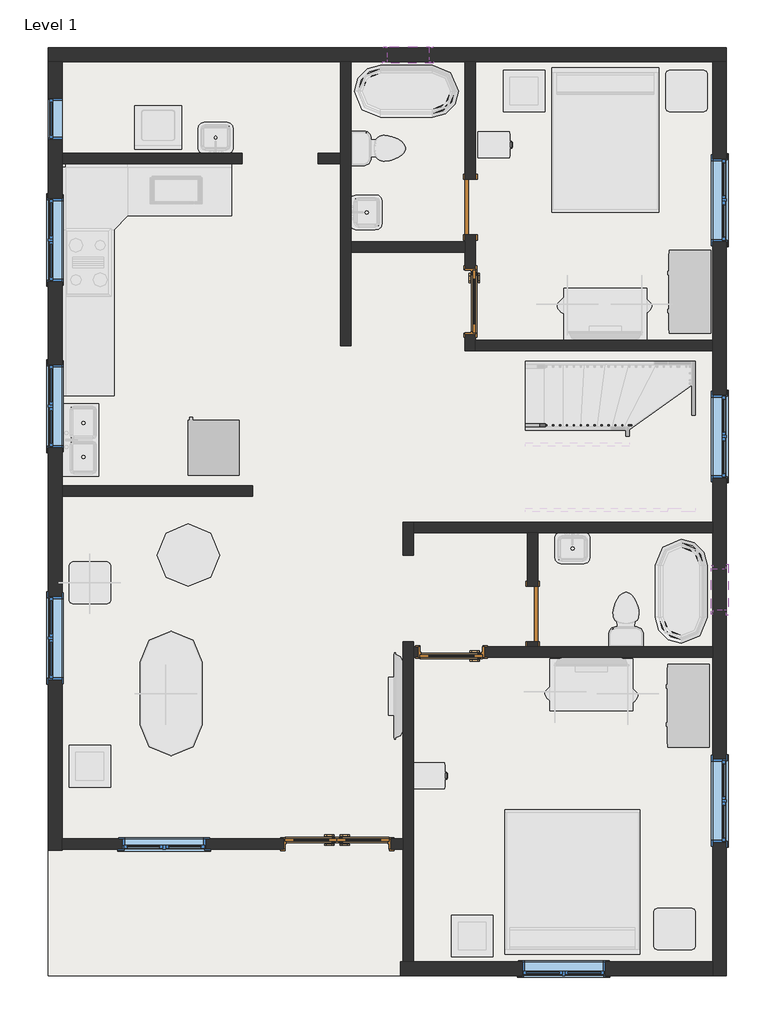
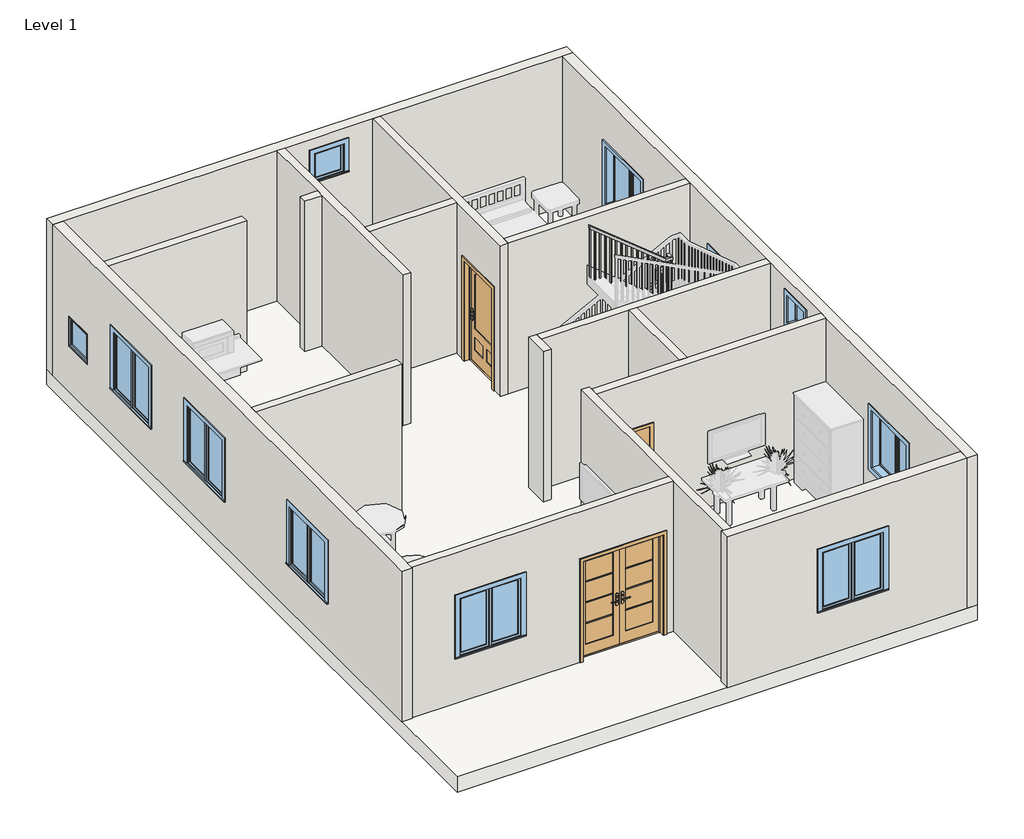
# One storey, part 1 of 2: 17 walls, 11 windows, 5 doors, 1 railing, 1 slab.
"""IFC4 building model written with IfcOpenShell, lengths in millimetres."""

from ifc_helpers import new_model, si_unit, frame, origin, origin_with_axes, place, context, project, spatial, polyline, outline, extrude, faceted_brep, transform, mapped, element, save
from components import door_5d363d20, door_94998e6c, door_377e7377, door_bb092f7c, window_0862ab64, window_be30da88, window_6846e476, window_e41d21a6

model = new_model("IFC4")

# Units and contexts
model_context = context("Model", 3, world=origin())
ifc_project = project(units=[si_unit("LENGTHUNIT", "METRE", prefix="MILLI")], contexts=[model_context])

# Site, building, storey
site = spatial("IfcSite", under=ifc_project)
building = spatial("IfcBuilding", under=site)
storey = spatial("IfcBuildingStorey", under=building, Name="Level 1", Elevation=0.0)

# Doors
placement = place(None, origin())
door_shape = door_5d363d20(model_context)
element("IfcDoor", 1, ObjectType="36\" x 80\"", at=placement, inside=storey, context=model_context, shape_type="MappedRepresentation", body=[
    mapped(door_shape, transform((-8609.4087964, 8043.0759458, 0.0), x_axis=(0.0, 1.0, 0.0), y_axis=(-1.0, 0.0, 0.0), z_axis=(0.0, 0.0, 1.0))),
])
element("IfcDoor", 2, ObjectType="36\" x 80\"", at=placement, inside=storey, context=model_context, shape_type="MappedRepresentation", body=[
    mapped(door_shape, transform((-8891.9837964, 2896.4009458, 0.0), x_axis=(1.0, 0.0, 0.0), y_axis=(0.0, 1.0, 0.0), z_axis=(0.0, 0.0, 1.0))),
])
door_2_shape = door_94998e6c(model_context)
element("IfcDoor", 3, ObjectType="Door-Exterior-Double-Full Glass-Wood_Clad : 60\" x 80\"", at=placement, inside=storey, context=model_context, shape_type="MappedRepresentation", body=[
    mapped(door_2_shape, transform((-10568.3837964, 83.3509458, 0.0), x_axis=(1.0, 0.0, 0.0), y_axis=(0.0, 1.0, 0.0), z_axis=(0.0, 0.0, 1.0))),
])
door_3_shape = door_377e7377(model_context)
element("IfcDoor", 4, ObjectType="Single-Flush : 32\" x 84\"", at=placement, inside=storey, context=model_context, shape_type="MappedRepresentation", body=[
    mapped(door_3_shape, transform((-7698.1837964, 3458.3759458, 0.0), x_axis=(0.0, -1.0, 0.0), y_axis=(1.0, 0.0, 0.0), z_axis=(0.0, 0.0, 1.0))),
])
door_4_shape = door_bb092f7c(model_context)
element("IfcDoor", 5, ObjectType="Single-Flush : 32\" x 84\"", at=placement, inside=storey, context=model_context, shape_type="MappedRepresentation", body=[
    mapped(door_4_shape, transform((-8612.5837964, 9427.3759458, 0.0), x_axis=(0.0, -1.0, 0.0), y_axis=(1.0, 0.0, 0.0), z_axis=(0.0, 0.0, 1.0))),
])

# Railing
element("IfcRailing", 6, ObjectType="Handrail - Rectangular", at=placement, inside=storey, context=model_context, shape_type="SolidModel", body=[
    faceted_brep([(-7803.5154882, 6252.3759458, 1025.2529681), (-7803.5154882, 6252.3759458, 959.7067088), (-7803.5154882, 6201.5759458, 959.7067088), (-7803.5154882, 6201.5759458, 1025.2529681), (-6351.9837964, 6252.3759458, 2208.7848338), (-6301.1837964, 6252.3759458, 2184.659247), (-6301.1837964, 6201.5759458, 2184.659247), (-6351.9837964, 6201.5759458, 2208.7848338), (-6351.9837964, 6252.3759458, 2414.6281882), (-6301.1837964, 6252.3759458, 2363.8281882), (-6301.1837964, 6201.5759458, 2363.8281882), (-6351.9837964, 6201.5759458, 2414.6281882), (-6224.9837964, 6252.3759458, 2414.6281882), (-6224.9837964, 6252.3759458, 2363.8281882), (-6275.7837964, 6201.5759458, 2363.8281882), (-6275.7837964, 6201.5759458, 2414.6281882), (-6224.9837964, 6125.3759458, 2414.6281882), (-6224.9837964, 6096.254612, 2363.8281882), (-6275.7837964, 6096.254612, 2363.8281882), (-6275.7837964, 6125.3759458, 2414.6281882), (-6224.9837964, 5998.3759458, 2631.5051451), (-6224.9837964, 5947.5759458, 2617.7256424), (-6275.7837964, 5947.5759458, 2617.7256424), (-6275.7837964, 5998.3759458, 2631.5051451), (-6224.9837964, 5998.3759458, 2837.3484995), (-6224.9837964, 5947.5759458, 2786.5484995), (-6275.7837964, 5947.5759458, 2786.5484995), (-6275.7837964, 5998.3759458, 2837.3484995), (-6224.9837964, 5871.3759458, 2837.3484995), (-6224.9837964, 5871.3759458, 2786.5484995), (-6275.7837964, 5922.1759458, 2786.5484995), (-6275.7837964, 5922.1759458, 2837.3484995), (-6351.9837964, 5871.3759458, 2837.3484995), (-6370.0692095, 5871.3759458, 2786.5484995), (-6370.0692095, 5922.1759458, 2786.5484995), (-6351.9837964, 5922.1759458, 2837.3484995), (-7803.5154882, 5871.3759458, 4020.8803652), (-7803.5154882, 5922.1759458, 4020.8803652), (-7803.5154882, 5922.1759458, 3955.3341059), (-7803.5154882, 5871.3759458, 3955.3341059)], [[[0, 1, 2, 3]], [[1, 0, 4, 5]], [[2, 1, 5, 6]], [[3, 2, 6, 7]], [[0, 3, 7, 4]], [[5, 4, 8, 9]], [[6, 5, 9, 10]], [[7, 6, 10, 11]], [[4, 7, 11, 8]], [[9, 8, 12, 13]], [[10, 9, 13, 14]], [[11, 10, 14, 15]], [[8, 11, 15, 12]], [[13, 12, 16, 17]], [[14, 13, 17, 18]], [[15, 14, 18, 19]], [[12, 15, 19, 16]], [[17, 16, 20, 21]], [[18, 17, 21, 22]], [[19, 18, 22, 23]], [[16, 19, 23, 20]], [[21, 20, 24, 25]], [[22, 21, 25, 26]], [[23, 22, 26, 27]], [[20, 23, 27, 24]], [[25, 24, 28, 29]], [[26, 25, 29, 30]], [[27, 26, 30, 31]], [[24, 27, 31, 28]], [[29, 28, 32, 33]], [[30, 29, 33, 34]], [[31, 30, 34, 35]], [[28, 31, 35, 32]], [[36, 37, 38, 39]], [[33, 32, 36, 39]], [[34, 33, 39, 38]], [[35, 34, 38, 37]], [[32, 35, 37, 36]]]),
    extrude(outline(polyline([(3866.2231262, -7694.2261527), (3881.7558784, -7713.2761527), (2878.6666667, -7713.2761527), (2878.6666667, -7694.2261527), (3866.2231262, -7694.2261527)])), frame((0.0, 5887.2509458, 0.0), z_axis=(0.0, 1.0, 0.0), x_axis=(0.0, 0.0, 1.0)), (0.0, 0.0, 1.0), 19.05),
    extrude(outline(polyline([(3783.3817813, -7592.6261527), (3798.9145334, -7611.6761527), (2878.6666667, -7611.6761527), (2878.6666667, -7592.6261527), (3783.3817813, -7592.6261527)])), frame((0.0, 5887.2509458, 0.0), z_axis=(0.0, 1.0, 0.0), x_axis=(0.0, 0.0, 1.0)), (0.0, 0.0, 1.0), 19.05),
    extrude(outline(polyline([(3700.5404364, -7491.0261527), (3716.0731885, -7510.0761527), (2709.3333333, -7510.0761527), (2709.3333333, -7491.0261527), (3700.5404364, -7491.0261527)])), frame((0.0, 5887.2509458, 0.0), z_axis=(0.0, 1.0, 0.0), x_axis=(0.0, 0.0, 1.0)), (0.0, 0.0, 1.0), 19.05),
    extrude(outline(polyline([(3617.6990914, -7389.4261527), (3633.2318436, -7408.4761527), (2709.3333333, -7408.4761527), (2709.3333333, -7389.4261527), (3617.6990914, -7389.4261527)])), frame((0.0, 5887.2509458, 0.0), z_axis=(0.0, 1.0, 0.0), x_axis=(0.0, 0.0, 1.0)), (0.0, 0.0, 1.0), 19.05),
    extrude(outline(polyline([(3534.8577465, -7287.8261527), (3550.3904987, -7306.8761527), (2709.3333333, -7306.8761527), (2709.3333333, -7287.8261527), (3534.8577465, -7287.8261527)])), frame((0.0, 5887.2509458, 0.0), z_axis=(0.0, 1.0, 0.0), x_axis=(0.0, 0.0, 1.0)), (0.0, 0.0, 1.0), 19.05),
    extrude(outline(polyline([(3452.0164016, -7186.2261527), (3467.5491538, -7205.2761527), (2540.0, -7205.2761527), (2540.0, -7186.2261527), (3452.0164016, -7186.2261527)])), frame((0.0, 5887.2509458, 0.0), z_axis=(0.0, 1.0, 0.0), x_axis=(0.0, 0.0, 1.0)), (0.0, 0.0, 1.0), 19.05),
    extrude(outline(polyline([(3369.1750567, -7084.6261527), (3384.7078088, -7103.6761527), (2540.0, -7103.6761527), (2540.0, -7084.6261527), (3369.1750567, -7084.6261527)])), frame((0.0, 5887.2509458, 0.0), z_axis=(0.0, 1.0, 0.0), x_axis=(0.0, 0.0, 1.0)), (0.0, 0.0, 1.0), 19.05),
    extrude(outline(polyline([(3286.3337117, -6983.0261527), (3301.8664639, -7002.0761527), (2540.0, -7002.0761527), (2540.0, -6983.0261527), (3286.3337117, -6983.0261527)])), frame((0.0, 5887.2509458, 0.0), z_axis=(0.0, 1.0, 0.0), x_axis=(0.0, 0.0, 1.0)), (0.0, 0.0, 1.0), 19.05),
    extrude(outline(polyline([(3203.4923668, -6881.4261527), (3219.025119, -6900.4761527), (2370.6666667, -6900.4761527), (2370.6666667, -6881.4261527), (3203.4923668, -6881.4261527)])), frame((0.0, 5887.2509458, 0.0), z_axis=(0.0, 1.0, 0.0), x_axis=(0.0, 0.0, 1.0)), (0.0, 0.0, 1.0), 19.05),
    extrude(outline(polyline([(3120.6510219, -6779.8261527), (3136.1837741, -6798.8761527), (2370.6666667, -6798.8761527), (2370.6666667, -6779.8261527), (3120.6510219, -6779.8261527)])), frame((0.0, 5887.2509458, 0.0), z_axis=(0.0, 1.0, 0.0), x_axis=(0.0, 0.0, 1.0)), (0.0, 0.0, 1.0), 19.05),
    extrude(outline(polyline([(3037.809677, -6678.2261527), (3053.3424291, -6697.2761527), (2201.3333333, -6697.2761527), (2201.3333333, -6678.2261527), (3037.809677, -6678.2261527)])), frame((0.0, 5887.2509458, 0.0), z_axis=(0.0, 1.0, 0.0), x_axis=(0.0, 0.0, 1.0)), (0.0, 0.0, 1.0), 19.05),
    extrude(outline(polyline([(2954.9683321, -6576.6261527), (2970.5010842, -6595.6761527), (2201.3333333, -6595.6761527), (2201.3333333, -6576.6261527), (2954.9683321, -6576.6261527)])), frame((0.0, 5887.2509458, 0.0), z_axis=(0.0, 1.0, 0.0), x_axis=(0.0, 0.0, 1.0)), (0.0, 0.0, 1.0), 19.05),
    extrude(outline(polyline([(2872.1269871, -6475.0261527), (2887.6597393, -6494.0761527), (2032.0, -6494.0761527), (2032.0, -6475.0261527), (2872.1269871, -6475.0261527)])), frame((0.0, 5887.2509458, 0.0), z_axis=(0.0, 1.0, 0.0), x_axis=(0.0, 0.0, 1.0)), (0.0, 0.0, 1.0), 19.05),
    extrude(outline(polyline([(2789.2856422, -6373.4261527), (2804.8183944, -6392.4761527), (2032.0, -6392.4761527), (2032.0, -6373.4261527), (2789.2856422, -6373.4261527)])), frame((0.0, 5887.2509458, 0.0), z_axis=(0.0, 1.0, 0.0), x_axis=(0.0, 0.0, 1.0)), (0.0, 0.0, 1.0), 19.05),
    extrude(outline(polyline([(5999.4650421, 2529.115018), (6018.5150421, 2496.5834745), (6018.5150421, 1524.0), (5999.4650421, 1524.0), (5999.4650421, 2529.115018)])), frame((-6259.9087964, 0.0, 0.0), z_axis=(1.0, 0.0, 0.0), x_axis=(0.0, 1.0, 0.0)), (0.0, 0.0, 1.0), 19.05),
    extrude(outline(polyline([(6101.0650421, 2355.6134525), (6120.1150421, 2323.0819089), (6120.1150421, 1524.0), (6101.0650421, 1524.0), (6101.0650421, 2355.6134525)])), frame((-6259.9087964, 0.0, 0.0), z_axis=(1.0, 0.0, 0.0), x_axis=(0.0, 1.0, 0.0)), (0.0, 0.0, 1.0), 19.05),
    extrude(outline(polyline([(2127.2519138, -6371.5904882), (2111.7191617, -6390.6404882), (1016.0, -6390.6404882), (1016.0, -6371.5904882), (2127.2519138, -6371.5904882)])), frame((0.0, 6217.4509458, 0.0), z_axis=(0.0, 1.0, 0.0), x_axis=(0.0, 0.0, 1.0)), (0.0, 0.0, 1.0), 19.05),
    extrude(outline(polyline([(2044.4105689, -6473.1904882), (2028.8778167, -6492.2404882), (1016.0, -6492.2404882), (1016.0, -6473.1904882), (2044.4105689, -6473.1904882)])), frame((0.0, 6217.4509458, 0.0), z_axis=(0.0, 1.0, 0.0), x_axis=(0.0, 0.0, 1.0)), (0.0, 0.0, 1.0), 19.05),
    extrude(outline(polyline([(1961.569224, -6574.7904882), (1946.0364718, -6593.8404882), (846.6666667, -6593.8404882), (846.6666667, -6574.7904882), (1961.569224, -6574.7904882)])), frame((0.0, 6217.4509458, 0.0), z_axis=(0.0, 1.0, 0.0), x_axis=(0.0, 0.0, 1.0)), (0.0, 0.0, 1.0), 19.05),
    extrude(outline(polyline([(1878.7278791, -6676.3904882), (1863.1951269, -6695.4404882), (846.6666667, -6695.4404882), (846.6666667, -6676.3904882), (1878.7278791, -6676.3904882)])), frame((0.0, 6217.4509458, 0.0), z_axis=(0.0, 1.0, 0.0), x_axis=(0.0, 0.0, 1.0)), (0.0, 0.0, 1.0), 19.05),
    extrude(outline(polyline([(1795.8865341, -6777.9904882), (1780.353782, -6797.0404882), (677.3333333, -6797.0404882), (677.3333333, -6777.9904882), (1795.8865341, -6777.9904882)])), frame((0.0, 6217.4509458, 0.0), z_axis=(0.0, 1.0, 0.0), x_axis=(0.0, 0.0, 1.0)), (0.0, 0.0, 1.0), 19.05),
    extrude(outline(polyline([(1713.0451892, -6879.5904882), (1697.5124371, -6898.6404882), (677.3333333, -6898.6404882), (677.3333333, -6879.5904882), (1713.0451892, -6879.5904882)])), frame((0.0, 6217.4509458, 0.0), z_axis=(0.0, 1.0, 0.0), x_axis=(0.0, 0.0, 1.0)), (0.0, 0.0, 1.0), 19.05),
    extrude(outline(polyline([(1630.2038443, -6981.1904882), (1614.6710921, -7000.2404882), (508.0, -7000.2404882), (508.0, -6981.1904882), (1630.2038443, -6981.1904882)])), frame((0.0, 6217.4509458, 0.0), z_axis=(0.0, 1.0, 0.0), x_axis=(0.0, 0.0, 1.0)), (0.0, 0.0, 1.0), 19.05),
    extrude(outline(polyline([(1547.3624994, -7082.7904882), (1531.8297472, -7101.8404882), (508.0, -7101.8404882), (508.0, -7082.7904882), (1547.3624994, -7082.7904882)])), frame((0.0, 6217.4509458, 0.0), z_axis=(0.0, 1.0, 0.0), x_axis=(0.0, 0.0, 1.0)), (0.0, 0.0, 1.0), 19.05),
    extrude(outline(polyline([(1464.5211545, -7184.3904882), (1448.9884023, -7203.4404882), (508.0, -7203.4404882), (508.0, -7184.3904882), (1464.5211545, -7184.3904882)])), frame((0.0, 6217.4509458, 0.0), z_axis=(0.0, 1.0, 0.0), x_axis=(0.0, 0.0, 1.0)), (0.0, 0.0, 1.0), 19.05),
    extrude(outline(polyline([(1381.6798095, -7285.9904882), (1366.1470574, -7305.0404882), (338.6666667, -7305.0404882), (338.6666667, -7285.9904882), (1381.6798095, -7285.9904882)])), frame((0.0, 6217.4509458, 0.0), z_axis=(0.0, 1.0, 0.0), x_axis=(0.0, 0.0, 1.0)), (0.0, 0.0, 1.0), 19.05),
    extrude(outline(polyline([(1298.8384646, -7387.5904882), (1283.3057124, -7406.6404882), (338.6666667, -7406.6404882), (338.6666667, -7387.5904882), (1298.8384646, -7387.5904882)])), frame((0.0, 6217.4509458, 0.0), z_axis=(0.0, 1.0, 0.0), x_axis=(0.0, 0.0, 1.0)), (0.0, 0.0, 1.0), 19.05),
    extrude(outline(polyline([(1215.9971197, -7489.1904882), (1200.4643675, -7508.2404882), (338.6666667, -7508.2404882), (338.6666667, -7489.1904882), (1215.9971197, -7489.1904882)])), frame((0.0, 6217.4509458, 0.0), z_axis=(0.0, 1.0, 0.0), x_axis=(0.0, 0.0, 1.0)), (0.0, 0.0, 1.0), 19.05),
    extrude(outline(polyline([(1133.1557748, -7590.7904882), (1117.6230226, -7609.8404882), (169.3333333, -7609.8404882), (169.3333333, -7590.7904882), (1133.1557748, -7590.7904882)])), frame((0.0, 6217.4509458, 0.0), z_axis=(0.0, 1.0, 0.0), x_axis=(0.0, 0.0, 1.0)), (0.0, 0.0, 1.0), 19.05),
    extrude(outline(polyline([(1050.3144298, -7692.3904882), (1034.7816777, -7711.4404882), (169.3333333, -7711.4404882), (169.3333333, -7692.3904882), (1050.3144298, -7692.3904882)])), frame((0.0, 6217.4509458, 0.0), z_axis=(0.0, 1.0, 0.0), x_axis=(0.0, 0.0, 1.0)), (0.0, 0.0, 1.0), 19.05),
    extrude(outline(polyline([(-6271.8261527, 5906.3009458), (-6271.8261527, 5887.2509458), (-6290.8761527, 5887.2509458), (-6290.8761527, 5906.3009458), (-6271.8261527, 5906.3009458)])), frame((0.0, 0.0, 1862.6666667), z_axis=(0.0, 0.0, 1.0), x_axis=(1.0, 0.0, 0.0)), (0.0, 0.0, 1.0), 923.8818329),
    extrude(outline(polyline([(-6259.9087964, 5906.3009458), (-6240.8587964, 5906.3009458), (-6240.8587964, 5887.2509458), (-6259.9087964, 5887.2509458), (-6259.9087964, 5906.3009458)])), frame((0.0, 0.0, 1862.6666667), z_axis=(0.0, 0.0, 1.0), x_axis=(1.0, 0.0, 0.0)), (0.0, 0.0, 1.0), 923.8818329),
    extrude(outline(polyline([(-6259.9087964, 5921.0868496), (-6240.8587964, 5921.0868496), (-6240.8587964, 5902.0368496), (-6259.9087964, 5902.0368496), (-6259.9087964, 5921.0868496)])), frame((0.0, 0.0, 1693.3333333), z_axis=(0.0, 0.0, 1.0), x_axis=(1.0, 0.0, 0.0)), (0.0, 0.0, 1.0), 1093.2151662),
    extrude(outline(polyline([(-6259.9087964, 6221.7150421), (-6240.8587964, 6221.7150421), (-6240.8587964, 6202.6650421), (-6259.9087964, 6202.6650421), (-6259.9087964, 6221.7150421)])), frame((0.0, 0.0, 1354.6666667), z_axis=(0.0, 0.0, 1.0), x_axis=(1.0, 0.0, 0.0)), (0.0, 0.0, 1.0), 1009.1615215),
    extrude(outline(polyline([(-6259.9087964, 6217.4509458), (-6259.9087964, 6236.5009458), (-6240.8587964, 6236.5009458), (-6240.8587964, 6217.4509458), (-6259.9087964, 6217.4509458)])), frame((0.0, 0.0, 1185.3333333), z_axis=(0.0, 0.0, 1.0), x_axis=(1.0, 0.0, 0.0)), (0.0, 0.0, 1.0), 1178.4948549),
    extrude(outline(polyline([(-6290.8761527, 6217.4509458), (-6290.8761527, 6236.5009458), (-6271.8261527, 6236.5009458), (-6271.8261527, 6217.4509458), (-6290.8761527, 6217.4509458)])), frame((0.0, 0.0, 1185.3333333), z_axis=(0.0, 0.0, 1.0), x_axis=(1.0, 0.0, 0.0)), (0.0, 0.0, 1.0), 1178.4948549),
    extrude(outline(polyline([(3939.8013537, -7784.4654882), (3955.3341059, -7803.5154882), (2878.6666667, -7803.5154882), (2878.6666667, -7784.4654882), (3939.8013537, -7784.4654882)])), frame((0.0, 5887.2509458, 0.0), z_axis=(0.0, 1.0, 0.0), x_axis=(0.0, 0.0, 1.0)), (0.0, 0.0, 1.0), 19.05),
    extrude(outline(polyline([(975.239461, -7784.4654882), (959.7067088, -7803.5154882), (169.3333333, -7803.5154882), (169.3333333, -7784.4654882), (975.239461, -7784.4654882)])), frame((0.0, 6217.4509458, 0.0), z_axis=(0.0, 1.0, 0.0), x_axis=(0.0, 0.0, 1.0)), (0.0, 0.0, 1.0), 19.05),
])

# Slab
element("IfcSlab", 7, ObjectType="Generic - 12\"", at=placement, inside=storey, context=model_context, shape_type="SweptSolid", body=[
    extrude(outline(polyline([(-4853.3837964, 11764.1759458), (-4853.3837964, -1850.2240542), (-14810.1837964, -1850.2240542), (-14810.1837964, 11764.1759458), (-4853.3837964, 11764.1759458)])), frame((0.0, 0.0, -304.8), z_axis=(0.0, 0.0, 1.0), x_axis=(1.0, 0.0, 0.0)), (0.0, 0.0, 1.0), 304.8),
])

# Walls
element("IfcWall", 8, ObjectType="Generic - 8\"", at=placement, inside=storey, context=model_context, shape_type="Brep", body=[
    faceted_brep([(-14810.1837964, 11560.9759458, 0.0), (-14606.9837964, 11560.9759458, 0.0), (-10517.5837964, 11560.9759458, 0.0), (-10365.1837964, 11560.9759458, 0.0), (-8688.7837964, 11560.9759458, 0.0), (-8536.3837964, 11560.9759458, 0.0), (-5056.5837964, 11560.9759458, 0.0), (-4853.3837964, 11560.9759458, 0.0), (-4853.3837964, 11560.9759458, 3048.0), (-5056.5837964, 11560.9759458, 3048.0), (-8536.3837964, 11560.9759458, 3048.0), (-8688.7837964, 11560.9759458, 3048.0), (-10365.1837964, 11560.9759458, 3048.0), (-10517.5837964, 11560.9759458, 3048.0), (-14606.9837964, 11560.9759458, 3048.0), (-14810.1837964, 11560.9759458, 3048.0), (-9831.7837964, 11560.9759458, 2768.6), (-9222.1837964, 11560.9759458, 2768.6), (-9222.1837964, 11560.9759458, 2159.0), (-9831.7837964, 11560.9759458, 2159.0), (-14810.1837964, 11764.1759458, 0.0), (-14810.1837964, 11764.1759458, 3048.0), (-4853.3837964, 11764.1759458, 3048.0), (-4853.3837964, 11764.1759458, 0.0), (-9831.7837964, 11764.1759458, 2768.6), (-9831.7837964, 11764.1759458, 2159.0), (-9222.1837964, 11764.1759458, 2159.0), (-9222.1837964, 11764.1759458, 2768.6)], [[[0, 1, 2, 3, 4, 5, 6, 7, 8, 9, 10, 11, 12, 13, 14, 15], [16, 17, 18, 19]], [[20, 21, 22, 23], [24, 25, 26, 27]], [[7, 6, 5, 4, 3, 2, 1, 0, 20, 23]], [[8, 7, 23, 22]], [[0, 15, 21, 20]], [[25, 24, 16, 19]], [[26, 25, 19, 18]], [[27, 26, 18, 17]], [[24, 27, 17, 16]], [[15, 14, 13, 12, 11, 10, 9, 8, 22, 21]]]),
])
element("IfcWall", 9, ObjectType="Generic - 8\"", at=placement, inside=storey, context=model_context, shape_type="Brep", body=[
    faceted_brep([(-5056.5837964, 11560.9759458, 0.0), (-5056.5837964, 7471.5759458, 0.0), (-5056.5837964, 7319.1759458, 0.0), (-5056.5837964, 4804.5759458, 0.0), (-5056.5837964, 4652.1759458, 0.0), (-5056.5837964, 2975.7759458, 0.0), (-5056.5837964, 2823.3759458, 0.0), (-5056.5837964, -1647.0240542, 0.0), (-5056.5837964, -1850.2240542, 0.0), (-5056.5837964, -1850.2240542, 3048.0), (-5056.5837964, -1647.0240542, 3048.0), (-5056.5837964, 2823.3759458, 3048.0), (-5056.5837964, 2975.7759458, 3048.0), (-5056.5837964, 4652.1759458, 3048.0), (-5056.5837964, 4804.5759458, 3048.0), (-5056.5837964, 7319.1759458, 3048.0), (-5056.5837964, 7471.5759458, 3048.0), (-5056.5837964, 11560.9759458, 3048.0), (-5056.5837964, 105.5759458, 2133.6), (-5056.5837964, 105.5759458, 914.4), (-5056.5837964, 1324.7759458, 914.4), (-5056.5837964, 1324.7759458, 2133.6), (-5056.5837964, 5452.2759458, 2133.6), (-5056.5837964, 5452.2759458, 914.4), (-5056.5837964, 6671.4759458, 914.4), (-5056.5837964, 6671.4759458, 2133.6), (-5056.5837964, 8919.3759458, 2133.6), (-5056.5837964, 8919.3759458, 914.4), (-5056.5837964, 10138.5759458, 914.4), (-5056.5837964, 10138.5759458, 2133.6), (-5056.5837964, 3509.1759458, 2768.6), (-5056.5837964, 3509.1759458, 2159.0), (-5056.5837964, 4118.7759458, 2159.0), (-5056.5837964, 4118.7759458, 2768.6), (-4853.3837964, 11560.9759458, 0.0), (-4853.3837964, 11560.9759458, 3048.0), (-4853.3837964, -1850.2240542, 3048.0), (-4853.3837964, -1850.2240542, 0.0), (-4853.3837964, 105.5759458, 2133.6), (-4853.3837964, 1324.7759458, 2133.6), (-4853.3837964, 1324.7759458, 914.4), (-4853.3837964, 105.5759458, 914.4), (-4853.3837964, 5452.2759458, 2133.6), (-4853.3837964, 6671.4759458, 2133.6), (-4853.3837964, 6671.4759458, 914.4), (-4853.3837964, 5452.2759458, 914.4), (-4853.3837964, 8919.3759458, 2133.6), (-4853.3837964, 10138.5759458, 2133.6), (-4853.3837964, 10138.5759458, 914.4), (-4853.3837964, 8919.3759458, 914.4), (-4853.3837964, 3509.1759458, 2768.6), (-4853.3837964, 4118.7759458, 2768.6), (-4853.3837964, 4118.7759458, 2159.0), (-4853.3837964, 3509.1759458, 2159.0)], [[[0, 1, 2, 3, 4, 5, 6, 7, 8, 9, 10, 11, 12, 13, 14, 15, 16, 17], [18, 19, 20, 21], [22, 23, 24, 25], [26, 27, 28, 29], [30, 31, 32, 33]], [[34, 35, 36, 37], [38, 39, 40, 41], [42, 43, 44, 45], [46, 47, 48, 49], [50, 51, 52, 53]], [[8, 7, 6, 5, 4, 3, 2, 1, 0, 34, 37]], [[0, 17, 35, 34]], [[9, 8, 37, 36]], [[19, 18, 38, 41]], [[20, 19, 41, 40]], [[21, 20, 40, 39]], [[18, 21, 39, 38]], [[23, 22, 42, 45]], [[24, 23, 45, 44]], [[25, 24, 44, 43]], [[22, 25, 43, 42]], [[27, 26, 46, 49]], [[28, 27, 49, 48]], [[29, 28, 48, 47]], [[26, 29, 47, 46]], [[31, 30, 50, 53]], [[32, 31, 53, 52]], [[33, 32, 52, 51]], [[30, 33, 51, 50]], [[17, 16, 15, 14, 13, 12, 11, 10, 9, 36, 35]]]),
])
element("IfcWall", 10, ObjectType="Generic - 8\"", at=placement, inside=storey, context=model_context, shape_type="Brep", body=[
    faceted_brep([(-5056.5837964, -1647.0240542, 0.0), (-9450.7837964, -1647.0240542, 0.0), (-9603.1837964, -1647.0240542, 0.0), (-9641.2837964, -1647.0240542, 0.0), (-9641.2837964, -1647.0240542, 3048.0), (-9603.1837964, -1647.0240542, 3048.0), (-9450.7837964, -1647.0240542, 3048.0), (-5056.5837964, -1647.0240542, 3048.0), (-7850.5837964, -1647.0240542, 2133.6), (-7850.5837964, -1647.0240542, 914.4), (-6631.3837964, -1647.0240542, 914.4), (-6631.3837964, -1647.0240542, 2133.6), (-5056.5837964, -1850.2240542, 0.0), (-5056.5837964, -1850.2240542, 3048.0), (-9641.2837964, -1850.2240542, 3048.0), (-9641.2837964, -1850.2240542, 0.0), (-7850.5837964, -1850.2240542, 2133.6), (-6631.3837964, -1850.2240542, 2133.6), (-6631.3837964, -1850.2240542, 914.4), (-7850.5837964, -1850.2240542, 914.4)], [[[0, 1, 2, 3, 4, 5, 6, 7], [8, 9, 10, 11]], [[12, 13, 14, 15], [16, 17, 18, 19]], [[3, 2, 1, 0, 12, 15]], [[4, 3, 15, 14]], [[0, 7, 13, 12]], [[9, 8, 16, 19]], [[10, 9, 19, 18]], [[11, 10, 18, 17]], [[8, 11, 17, 16]], [[7, 6, 5, 4, 14, 13]]]),
])
element("IfcWall", 11, ObjectType="Generic - 8\"", at=placement, inside=storey, context=model_context, shape_type="Brep", body=[
    faceted_brep([(-14606.9837964, -8.7240542, 0.0), (-14606.9837964, 3.9759458, 0.0), (-14606.9837964, 156.3759458, 0.0), (-14606.9837964, 5185.5759458, 0.0), (-14606.9837964, 5337.9759458, 0.0), (-14606.9837964, 10062.3759458, 0.0), (-14606.9837964, 10214.7759458, 0.0), (-14606.9837964, 11560.9759458, 0.0), (-14606.9837964, 11560.9759458, 3048.0), (-14606.9837964, 10214.7759458, 3048.0), (-14606.9837964, 10062.3759458, 3048.0), (-14606.9837964, 5337.9759458, 3048.0), (-14606.9837964, 5185.5759458, 3048.0), (-14606.9837964, 156.3759458, 3048.0), (-14606.9837964, 3.9759458, 3048.0), (-14606.9837964, -8.7240542, 3048.0), (-14606.9837964, 9554.3759458, 2133.6), (-14606.9837964, 9554.3759458, 914.4), (-14606.9837964, 8335.1759458, 914.4), (-14606.9837964, 8335.1759458, 2133.6), (-14606.9837964, 7115.9759458, 2133.6), (-14606.9837964, 7115.9759458, 914.4), (-14606.9837964, 5896.7759458, 914.4), (-14606.9837964, 5896.7759458, 2133.6), (-14606.9837964, 3712.3759458, 2133.6), (-14606.9837964, 3712.3759458, 914.4), (-14606.9837964, 2493.1759458, 914.4), (-14606.9837964, 2493.1759458, 2133.6), (-14606.9837964, 11027.5759458, 1524.0), (-14606.9837964, 11027.5759458, 914.4), (-14606.9837964, 10417.9759458, 914.4), (-14606.9837964, 10417.9759458, 1524.0), (-14810.1837964, -8.7240542, 0.0), (-14810.1837964, -8.7240542, 3048.0), (-14810.1837964, 11560.9759458, 3048.0), (-14810.1837964, 11560.9759458, 0.0), (-14810.1837964, 9554.3759458, 2133.6), (-14810.1837964, 8335.1759458, 2133.6), (-14810.1837964, 8335.1759458, 914.4), (-14810.1837964, 9554.3759458, 914.4), (-14810.1837964, 7115.9759458, 2133.6), (-14810.1837964, 5896.7759458, 2133.6), (-14810.1837964, 5896.7759458, 914.4), (-14810.1837964, 7115.9759458, 914.4), (-14810.1837964, 3712.3759458, 2133.6), (-14810.1837964, 2493.1759458, 2133.6), (-14810.1837964, 2493.1759458, 914.4), (-14810.1837964, 3712.3759458, 914.4), (-14810.1837964, 11027.5759458, 1524.0), (-14810.1837964, 10417.9759458, 1524.0), (-14810.1837964, 10417.9759458, 914.4), (-14810.1837964, 11027.5759458, 914.4)], [[[0, 1, 2, 3, 4, 5, 6, 7, 8, 9, 10, 11, 12, 13, 14, 15], [16, 17, 18, 19], [20, 21, 22, 23], [24, 25, 26, 27], [28, 29, 30, 31]], [[32, 33, 34, 35], [36, 37, 38, 39], [40, 41, 42, 43], [44, 45, 46, 47], [48, 49, 50, 51]], [[7, 6, 5, 4, 3, 2, 1, 0, 32, 35]], [[0, 15, 33, 32]], [[8, 7, 35, 34]], [[17, 16, 36, 39]], [[18, 17, 39, 38]], [[19, 18, 38, 37]], [[16, 19, 37, 36]], [[21, 20, 40, 43]], [[22, 21, 43, 42]], [[23, 22, 42, 41]], [[20, 23, 41, 40]], [[25, 24, 44, 47]], [[26, 25, 47, 46]], [[27, 26, 46, 45]], [[24, 27, 45, 44]], [[29, 28, 48, 51]], [[30, 29, 51, 50]], [[31, 30, 50, 49]], [[28, 31, 49, 48]], [[15, 14, 13, 12, 11, 10, 9, 8, 34, 33]]]),
])
element("IfcWall", 12, ObjectType="INNER 6\"", at=placement, inside=storey, context=model_context, shape_type="SweptSolid", body=[
    extrude(outline(polyline([(-11965.3837964, 10062.3759458), (-14606.9837964, 10062.3759458), (-14606.9837964, 10214.7759458), (-11965.3837964, 10214.7759458), (-11965.3837964, 10062.3759458)])), origin_with_axes(), (0.0, 0.0, 1.0), 3048.0),
])
element("IfcWall", 13, ObjectType="INNER 6\"", at=placement, inside=storey, context=model_context, shape_type="Brep", body=[
    faceted_brep([(-8688.7837964, 9020.9759458, 2133.6), (-8688.7837964, 9020.9759458, 0.0), (-8688.7837964, 8919.3759458, 0.0), (-8688.7837964, 8766.9759458, 0.0), (-8688.7837964, 8525.6759458, 0.0), (-8688.7837964, 8525.6759458, 2057.4), (-8688.7837964, 7560.4759458, 2057.4), (-8688.7837964, 7560.4759458, 0.0), (-8688.7837964, 7319.1759458, 0.0), (-8688.7837964, 7319.1759458, 3048.0), (-8688.7837964, 8766.9759458, 3048.0), (-8688.7837964, 8919.3759458, 3048.0), (-8688.7837964, 11560.9759458, 3048.0), (-8688.7837964, 11560.9759458, 0.0), (-8688.7837964, 9833.7759458, 0.0), (-8688.7837964, 9833.7759458, 2133.6), (-8536.3837964, 8525.6759458, 0.0), (-8536.3837964, 9020.9759458, 0.0), (-8536.3837964, 9020.9759458, 2133.6), (-8536.3837964, 9833.7759458, 2133.6), (-8536.3837964, 9833.7759458, 0.0), (-8536.3837964, 11560.9759458, 0.0), (-8536.3837964, 11560.9759458, 3048.0), (-8536.3837964, 7471.5759458, 3048.0), (-8536.3837964, 7319.1759458, 3048.0), (-8536.3837964, 7319.1759458, 0.0), (-8536.3837964, 7471.5759458, 0.0), (-8536.3837964, 7560.4759458, 0.0), (-8536.3837964, 7560.4759458, 2057.4), (-8536.3837964, 8525.6759458, 2057.4)], [[[0, 1, 2, 3, 4, 5, 6, 7, 8, 9, 10, 11, 12, 13, 14, 15]], [[16, 17, 18, 19, 20, 21, 22, 23, 24, 25, 26, 27, 28, 29]], [[25, 8, 7, 27, 26]], [[14, 13, 21, 20]], [[4, 3, 2, 1, 17, 16]], [[13, 12, 22, 21]], [[9, 8, 25, 24]], [[29, 5, 4, 16]], [[5, 29, 28, 6]], [[6, 28, 27, 7]], [[18, 17, 1, 0]], [[19, 18, 0, 15]], [[20, 19, 15, 14]], [[12, 11, 10, 9, 24, 23, 22]]]),
])
element("IfcWall", 14, ObjectType="INNER 6\"", at=placement, inside=storey, context=model_context, shape_type="SweptSolid", body=[
    extrude(outline(polyline([(-5056.5837964, 7319.1759458), (-8536.3837964, 7319.1759458), (-8536.3837964, 7471.5759458), (-5056.5837964, 7471.5759458), (-5056.5837964, 7319.1759458)])), origin_with_axes(), (0.0, 0.0, 1.0), 3048.0),
])
element("IfcWall", 15, ObjectType="INNER 6\"", at=placement, inside=storey, context=model_context, shape_type="SweptSolid", body=[
    extrude(outline(polyline([(-10365.1837964, 8919.3759458), (-8688.7837964, 8919.3759458), (-8688.7837964, 8766.9759458), (-10365.1837964, 8766.9759458), (-10365.1837964, 8919.3759458)])), origin_with_axes(), (0.0, 0.0, 1.0), 3048.0),
])
element("IfcWall", 16, ObjectType="INNER 6\"", at=placement, inside=storey, context=model_context, shape_type="Brep", body=[
    faceted_brep([(-10365.1837964, 7395.3759458, 0.0), (-10365.1837964, 8766.9759458, 0.0), (-10365.1837964, 8919.3759458, 0.0), (-10365.1837964, 11560.9759458, 0.0), (-10365.1837964, 11560.9759458, 3048.0), (-10365.1837964, 8919.3759458, 3048.0), (-10365.1837964, 8766.9759458, 3048.0), (-10365.1837964, 7395.3759458, 3048.0), (-10517.5837964, 7395.3759458, 0.0), (-10517.5837964, 7395.3759458, 3048.0), (-10517.5837964, 10062.3759458, 3048.0), (-10517.5837964, 10214.7759458, 3048.0), (-10517.5837964, 11560.9759458, 3048.0), (-10517.5837964, 11560.9759458, 0.0), (-10517.5837964, 10214.7759458, 0.0), (-10517.5837964, 10062.3759458, 0.0)], [[[0, 1, 2, 3, 4, 5, 6, 7]], [[8, 9, 10, 11, 12, 13, 14, 15]], [[3, 2, 1, 0, 8, 15, 14, 13]], [[0, 7, 9, 8]], [[4, 3, 13, 12]], [[7, 6, 5, 4, 12, 11, 10, 9]]]),
])
element("IfcWall", 17, ObjectType="INNER 6\"", at=placement, inside=storey, context=model_context, shape_type="SweptSolid", body=[
    extrude(outline(polyline([(-14606.9837964, 5337.9759458), (-11812.9837964, 5337.9759458), (-11812.9837964, 5185.5759458), (-14606.9837964, 5185.5759458), (-14606.9837964, 5337.9759458)])), origin_with_axes(), (0.0, 0.0, 1.0), 3048.0),
])
element("IfcWall", 18, ObjectType="INNER 6\"", at=placement, inside=storey, context=model_context, shape_type="SweptSolid", body=[
    extrude(outline(polyline([(3048.0, -14606.9837964), (0.0, -14606.9837964), (0.0, -11355.7837964), (2057.4, -11355.7837964), (2057.4, -9780.9837964), (0.0, -9780.9837964), (0.0, -9603.1837964), (3048.0, -9603.1837964), (3048.0, -14606.9837964)]), holes=[polyline([(2133.6, -13717.9837964), (2133.6, -12498.7837964), (914.4, -12498.7837964), (914.4, -13717.9837964), (2133.6, -13717.9837964)])]), frame((0.0, 3.9759458, 0.0), z_axis=(0.0, 1.0, 0.0), x_axis=(0.0, 0.0, 1.0)), (0.0, 0.0, 1.0), 152.4),
])
element("IfcWall", 19, ObjectType="INNER 6\"", at=placement, inside=storey, context=model_context, shape_type="Brep", body=[
    faceted_brep([(-9450.7837964, -1647.0240542, 0.0), (-9450.7837964, 2823.3759458, 0.0), (-9450.7837964, 2975.7759458, 0.0), (-9450.7837964, 3051.9759458, 0.0), (-9450.7837964, 3051.9759458, 3048.0), (-9450.7837964, 2975.7759458, 3048.0), (-9450.7837964, 2823.3759458, 3048.0), (-9450.7837964, -1647.0240542, 3048.0), (-9603.1837964, -1647.0240542, 0.0), (-9603.1837964, -1647.0240542, 3048.0), (-9603.1837964, 3.9759458, 3048.0), (-9603.1837964, 156.3759458, 3048.0), (-9603.1837964, 3051.9759458, 3048.0), (-9603.1837964, 3051.9759458, 0.0), (-9603.1837964, 156.3759458, 0.0), (-9603.1837964, 3.9759458, 0.0)], [[[0, 1, 2, 3, 4, 5, 6, 7]], [[8, 9, 10, 11, 12, 13, 14, 15]], [[3, 2, 1, 0, 8, 15, 14, 13]], [[4, 3, 13, 12]], [[0, 7, 9, 8]], [[7, 6, 5, 4, 12, 11, 10, 9]]]),
])
element("IfcWall", 20, ObjectType="INNER 6\"", at=placement, inside=storey, context=model_context, shape_type="Brep", body=[
    faceted_brep([(-9450.7837964, 4652.1759458, 0.0), (-7774.3837964, 4652.1759458, 0.0), (-7621.9837964, 4652.1759458, 0.0), (-5056.5837964, 4652.1759458, 0.0), (-5056.5837964, 4652.1759458, 3048.0), (-7621.9837964, 4652.1759458, 3048.0), (-7774.3837964, 4652.1759458, 3048.0), (-9450.7837964, 4652.1759458, 3048.0), (-9450.7837964, 4804.5759458, 0.0), (-9450.7837964, 4804.5759458, 3048.0), (-5056.5837964, 4804.5759458, 3048.0), (-5056.5837964, 4804.5759458, 0.0)], [[[0, 1, 2, 3, 4, 5, 6, 7]], [[8, 9, 10, 11]], [[3, 2, 1, 0, 8, 11]], [[0, 7, 9, 8]], [[4, 3, 11, 10]], [[7, 6, 5, 4, 10, 9]]]),
])
element("IfcWall", 21, ObjectType="INNER 6\"", at=placement, inside=storey, context=model_context, shape_type="Brep", body=[
    faceted_brep([(-5056.5837964, 2823.3759458, 0.0), (-5056.5837964, 2823.3759458, 3048.0), (-9450.7837964, 2823.3759458, 3048.0), (-9450.7837964, 2823.3759458, 0.0), (-9374.5837964, 2823.3759458, 0.0), (-9374.5837964, 2823.3759458, 2057.4), (-8409.3837964, 2823.3759458, 2057.4), (-8409.3837964, 2823.3759458, 0.0), (-5056.5837964, 2975.7759458, 3048.0), (-5056.5837964, 2975.7759458, 0.0), (-7621.9837964, 2975.7759458, 0.0), (-7774.3837964, 2975.7759458, 0.0), (-8409.3837964, 2975.7759458, 0.0), (-8409.3837964, 2975.7759458, 2057.4), (-9374.5837964, 2975.7759458, 2057.4), (-9374.5837964, 2975.7759458, 0.0), (-9450.7837964, 2975.7759458, 0.0), (-9450.7837964, 2975.7759458, 3048.0), (-7774.3837964, 2975.7759458, 3048.0), (-7621.9837964, 2975.7759458, 3048.0)], [[[0, 1, 2, 3, 4, 5, 6, 7]], [[8, 9, 10, 11, 12, 13, 14, 15, 16, 17, 18, 19]], [[3, 16, 15, 4]], [[9, 0, 7, 12, 11, 10]], [[1, 0, 9, 8]], [[3, 2, 17, 16]], [[6, 13, 12, 7]], [[13, 6, 5, 14]], [[14, 5, 4, 15]], [[2, 1, 8, 19, 18, 17]]]),
])
element("IfcWall", 22, ObjectType="INNER 6\"", at=placement, inside=storey, context=model_context, shape_type="SweptSolid", body=[
    extrude(outline(polyline([(3051.9759458, 2133.6), (3051.9759458, 0.0), (2975.7759458, 0.0), (2975.7759458, 3048.0), (4652.1759458, 3048.0), (4652.1759458, 0.0), (3864.7759458, 0.0), (3864.7759458, 2133.6), (3051.9759458, 2133.6)])), frame((-7774.3837964, 0.0, 0.0), z_axis=(1.0, 0.0, 0.0), x_axis=(0.0, 1.0, 0.0)), (0.0, 0.0, 1.0), 152.4),
])
element("IfcWall", 23, ObjectType="INNER 6\"", at=placement, inside=storey, context=model_context, shape_type="Brep", body=[
    faceted_brep([(-9450.7837964, 4321.9759458, 0.0), (-9450.7837964, 4652.1759458, 0.0), (-9450.7837964, 4804.5759458, 0.0), (-9450.7837964, 4804.5759458, 3048.0), (-9450.7837964, 4652.1759458, 3048.0), (-9450.7837964, 4321.9759458, 3048.0), (-9603.1837964, 4321.9759458, 0.0), (-9603.1837964, 4321.9759458, 3048.0), (-9603.1837964, 4804.5759458, 3048.0), (-9603.1837964, 4804.5759458, 0.0)], [[[0, 1, 2, 3, 4, 5]], [[6, 7, 8, 9]], [[2, 1, 0, 6, 9]], [[0, 5, 7, 6]], [[3, 2, 9, 8]], [[5, 4, 3, 8, 7]]]),
])
element("IfcWall", 24, ObjectType="INNER 6\"", at=placement, inside=storey, context=model_context, shape_type="SweptSolid", body=[
    extrude(outline(polyline([(-10517.5837964, 10062.3759458), (-10847.7837964, 10062.3759458), (-10847.7837964, 10214.7759458), (-10517.5837964, 10214.7759458), (-10517.5837964, 10062.3759458)])), origin_with_axes(), (0.0, 0.0, 1.0), 3048.0),
])

# Windows
window_shape = window_0862ab64(model_context)
element("IfcWindow", 25, ObjectType="Casement Dbl with Trim : 48\" x 48\"", at=placement, inside=storey, context=model_context, shape_type="MappedRepresentation", body=[
    mapped(window_shape, transform((-14689.5337964, 8944.7759458, 0.0), x_axis=(0.0, 1.0, 0.0), y_axis=(-1.0, 0.0, 0.0), z_axis=(0.0, 0.0, 1.0))),
])
element("IfcWindow", 26, ObjectType="Casement Dbl with Trim : 48\" x 48\"", at=placement, inside=storey, context=model_context, shape_type="MappedRepresentation", body=[
    mapped(window_shape, transform((-14689.5337964, 6506.3759458, 0.0), x_axis=(0.0, 1.0, 0.0), y_axis=(-1.0, 0.0, 0.0), z_axis=(0.0, 0.0, 1.0))),
])
element("IfcWindow", 27, ObjectType="Casement Dbl with Trim : 48\" x 48\"", at=placement, inside=storey, context=model_context, shape_type="MappedRepresentation", body=[
    mapped(window_shape, transform((-14689.5337964, 3102.7759458, 0.0), x_axis=(0.0, 1.0, 0.0), y_axis=(-1.0, 0.0, 0.0), z_axis=(0.0, 0.0, 1.0))),
])
element("IfcWindow", 28, ObjectType="Casement Dbl with Trim : 48\" x 48\"", at=placement, inside=storey, context=model_context, shape_type="MappedRepresentation", body=[
    mapped(window_shape, transform((-7240.9837964, -1729.5740542, 0.0), x_axis=(-1.0, 0.0, 0.0), y_axis=(0.0, -1.0, 0.0), z_axis=(0.0, 0.0, 1.0))),
])
element("IfcWindow", 29, ObjectType="Casement Dbl with Trim : 48\" x 48\"", at=placement, inside=storey, context=model_context, shape_type="MappedRepresentation", body=[
    mapped(window_shape, transform((-4974.0337964, 715.1759458, 0.0), x_axis=(0.0, -1.0, 0.0), y_axis=(1.0, 0.0, 0.0), z_axis=(0.0, 0.0, 1.0))),
])
element("IfcWindow", 30, ObjectType="Casement Dbl with Trim : 48\" x 48\"", at=placement, inside=storey, context=model_context, shape_type="MappedRepresentation", body=[
    mapped(window_shape, transform((-4974.0337964, 6061.8759458, 0.0), x_axis=(0.0, -1.0, 0.0), y_axis=(1.0, 0.0, 0.0), z_axis=(0.0, 0.0, 1.0))),
])
element("IfcWindow", 31, ObjectType="Casement Dbl with Trim : 48\" x 48\"", at=placement, inside=storey, context=model_context, shape_type="MappedRepresentation", body=[
    mapped(window_shape, transform((-4974.0337964, 9528.9759458, 0.0), x_axis=(0.0, -1.0, 0.0), y_axis=(1.0, 0.0, 0.0), z_axis=(0.0, 0.0, 1.0))),
])
window_2_shape = window_be30da88(model_context)
element("IfcWindow", 32, ObjectType="Casement Dbl with Trim : 48\" x 48\"", at=placement, inside=storey, context=model_context, shape_type="MappedRepresentation", body=[
    mapped(window_2_shape, transform((-13108.3837964, 99.2259458, 0.0), x_axis=(-1.0, 0.0, 0.0), y_axis=(0.0, -1.0, 0.0), z_axis=(0.0, 0.0, 1.0))),
])
window_3_shape = window_6846e476(model_context)
element("IfcWindow", 33, ObjectType="Fixed : 24\" x 24\"", at=placement, inside=storey, context=model_context, shape_type="MappedRepresentation", body=[
    mapped(window_3_shape, transform((-14708.5837964, 10760.8759458, 0.0), x_axis=(0.0, 1.0, 0.0), y_axis=(-1.0, 0.0, 0.0), z_axis=(0.0, 0.0, 1.0))),
])
window_4_shape = window_e41d21a6(model_context)
element("IfcWindow", 34, ObjectType="Transom with Trim : 24\" x 24\"", at=placement, inside=storey, context=model_context, shape_type="MappedRepresentation", body=[
    mapped(window_4_shape, transform((-9565.0837964, 11662.5759458, 0.0), x_axis=(-1.0, 0.0, 0.0), y_axis=(0.0, -1.0, 0.0), z_axis=(0.0, 0.0, 1.0))),
])
element("IfcWindow", 35, ObjectType="Transom with Trim : 24\" x 24\"", at=placement, inside=storey, context=model_context, shape_type="MappedRepresentation", body=[
    mapped(window_4_shape, transform((-4954.9837964, 3775.8759458, 0.0), x_axis=(0.0, -1.0, 0.0), y_axis=(1.0, 0.0, 0.0), z_axis=(0.0, 0.0, 1.0))),
])

save(model, "model.ifc")

# Revit data of these elements
# Type "36\" x 80\""
#   Type Mark = "8"
#   Assembly Code = "B2030100"
#   Analytic Construction = "French door, wood frame with single glass"
#   Threshold Offset [instance default] = 0' - 0 1/2"
#   Thickness = 0' - 1 3/8"
#   Thermal Resistance (R) = 1.0696 (h·ft²·°F)/BTU
#   Swing Angle [instance default] = 90.00°
#   Stiles = 0' - 4 3/4"
#   Rough Width = 3' - 2"
#   Rough Height = 6' - 9"
#   Radius = 1' - 8.05625"
#   Lock Rail = 0' - 7 1/8"
#   Height = 6' - 8"
#   Width = 3' - 0"
#   Heat Transfer Coefficient (U) = 0.9350 BTU/(h·ft²·°F)
#   Door Offset [instance default] = 0' - 0"
#   Bottom Rail = 0' - 9 1/2"
#   Threshold [instance default] = yes
#   Function = 1
#   Exterior Trim [instance default] = yes
#   Trim Material = Cherry
#   Threshold Material = Cherry
#   Panel Material = Cherry
#   Glazing = Glass
#   Frame Material = Cherry
#   Door Handle Material = Aluminum
#   Visual Light Transmittance = 0
#   Solar Heat Gain Coefficient = 0
#   Wall Closure = (empty or 0)
#   Construction Type = (empty or 0)
# Type "Door-Exterior-Double-Full Glass-Wood_Clad : 60\" x 80\""
#   Type Mark = "9"
#   Assembly Code = "B2030100"
#   Analytic Construction = "French door, wood frame with double glass"
#   Top Rail = 0' - 4 11/16"
#   Threshold Offset [instance default] = 0' - 0 1/2"
#   Thickness = 0' - 1 3/8"
#   Thermal Resistance (R) = 1.9158 (h·ft²·°F)/BTU
#   Swing Angle [instance default] = 90.00°
#   Stiles = 0' - 4 3/4"
#   Rough Width = 5' - 2"
#   Rough Height = 6' - 9"
#   Panel Width = 2' - 6"
#   Door Offset [instance default] = 0' - 0"
#   Height = 6' - 8"
#   Width = 5' - 0"
#   Heat Transfer Coefficient (U) = 0.5220 BTU/(h·ft²·°F)
#   Bottom Rail = 0' - 9 1/8"
#   Exterior Trim [instance default] = yes
#   Threshold [instance default] = yes
#   Show Grill [instance default] = yes
#   Function = 1
#   Trim Material = Cherry
#   Threshold Material = Cherry
#   Panel Material = Cherry
#   Glazing = Glass
#   Frame Material = Cherry
#   Door Handle Material = Aluminum
#   Visual Light Transmittance = 0
#   Solar Heat Gain Coefficient = 0
#   Wall Closure = (empty or 0)
#   Construction Type = (empty or 0)
# Type "Single-Flush : 32\" x 84\""
#   Type Mark = "3"
#   Construction Type Id = "MDOOR"
#   Assembly Code = "C1020"
#   Analytic Construction = "Metal"
#   Thickness = 0' - 2"
#   Heat Transfer Coefficient (U) = 0.651978 BTU/(h·ft²·°F)
#   Height = 7' - 0"
#   Trim Projection Ext = 0' - 1"
#   Trim Projection Int = 0' - 1"
#   Trim Width = 0' - 3"
#   Width = 2' - 8"
#   Define Thermal Properties by = 1
#   Door Material = Door - Panel
#   Frame Material = Door - Frame
#   Visual Light Transmittance = 0
#   Solar Heat Gain Coefficient = 0
#   Function = (empty or 0)
#   Wall Closure = (empty or 0)
# Type "Handrail - Rectangular"
#   Assembly Code = "C2010400"
#   built-in parameter 1008612 = 0.0416667 (stored number, unit not read)
#   built-in parameter 1008611 = 0.0416667 (stored number, unit not read)
#   built-in parameter 1008609 = 0.333333 (stored number, unit not read)
#   built-in parameter 1008604 = 0.166667 (stored number, unit not read)
#   built-in parameter 1008603 = 0.166667 (stored number, unit not read)
#   Railing Height = 3' - 0"
#   built-in parameter 1008630 = 2
#   built-in parameter 1008610 = 2
#   built-in parameter 1008618 = Baluster - Square : 3/4"
# Type "Generic - 12\""
#   Assembly Code = "B1010"
#   Function = 0
#   Layers, outside or top first: 1' - 0" no material (function 1)
# Type "Generic - 8\""
#   Assembly Code = "B2010"
#   Layers, outside or top first: 0' - 8" "Brick, Common" (function 1)
# Type "INNER 6\""
#   Assembly Code = "B2010"
#   Layers, outside or top first: 0' - 6" "Brick, Common" (function 1)
# Type "Casement Dbl with Trim : 48\" x 48\""
#   Type Mark = "10"
#   Construction Type Id = "GSP4R"
#   Assembly Code = "B2020100"
#   Analytic Construction = "1/8 in Pilkington single glazing"
#   Visual Light Transmittance = 0.9
#   Solar Heat Gain Coefficient = 0.78
#   Heat Transfer Coefficient (U) = 0.6496 BTU/(h·ft²·°F)
#   Height = 4' - 0"
#   Default Sill Height = 3' - 0"
#   Trim Projection - Ext. = 0' - 0 1/2"
#   Trim Projection - Int. = 0' - 0 3/4"
#   Trim Width - Exterior = 0' - 3 1/2"
#   Trim Width - Interior = 0' - 3 1/2"
#   Width = 4' - 0"
#   Window Inset = 0' - 0 3/4"
#   Define Thermal Properties by = 1
#   Glass Pane Material = Glass
#   Sash Material = Sash
#   Trim Exterior Material = Trim
#   Trim Interior Material = Trim
#   Wall Closure = (empty or 0)
# Type "Fixed : 24\" x 24\""
#   Type Mark = "3"
#   Construction Type Id = "GSP4R"
#   Assembly Code = "B2020100"
#   Analytic Construction = "1/8 in Pilkington single glazing"
#   Visual Light Transmittance = 0.9
#   Solar Heat Gain Coefficient = 0.78
#   Heat Transfer Coefficient (U) = 0.6496 BTU/(h·ft²·°F)
#   Height = 2' - 0"
#   Default Sill Height = 3' - 0"
#   Width = 2' - 0"
#   Window Inset = 0' - 0 3/4"
#   Define Thermal Properties by = 1
#   Glass Pane Material = Glass
#   Sash Material = Sash
#   Wall Closure = (empty or 0)
# Type "Transom with Trim : 24\" x 24\""
#   Type Mark = "13"
#   Construction Type Id = "GSP4R"
#   Assembly Code = "B2020100"
#   Analytic Construction = "1/8 in Pilkington single glazing"
#   Visual Light Transmittance = 0.9
#   Solar Heat Gain Coefficient = 0.78
#   Heat Transfer Coefficient (U) = 0.6496 BTU/(h·ft²·°F)
#   Height = 2' - 0"
#   Default Sill Height = 7' - 1"
#   Trim Projection - Ext. = 0' - 0 1/2"
#   Trim Projection - Int. = 0' - 0 3/4"
#   Trim Width - Exterior = 0' - 3 1/2"
#   Trim Width - Interior = 0' - 3 1/2"
#   Width = 2' - 0"
#   Window Inset = 0' - 0 3/4"
#   Define Thermal Properties by = 1
#   Glass Pane Material = Glass
#   Sash Material = Sash
#   Trim Exterior Material = Trim
#   Trim Interior Material = Trim
#   Wall Closure = (empty or 0)
# Elements 1, 2 (IfcDoor, "36\" x 80\"")
#   Threshold Offset = 0' - 0 1/2"
#   Swing Angle = 90.00°
#   Door Offset = 0' - 0"
#   Threshold = yes
#   Exterior Trim = yes
#   Phase Created = New Construction
#   Materials on its faces: "Cherry", "Aluminum", "Glass"
# Element 3 (IfcDoor, "Door-Exterior-Double-Full Glass-Wood_Clad : 60\" x 80\"")
#   Threshold Offset = 0' - 0 1/2"
#   Swing Angle = 90.00°
#   Door Offset = 0' - 0"
#   Threshold = yes
#   Show Grill = yes
#   Exterior Trim = yes
#   Phase Created = New Construction
#   Materials on its faces: "Cherry", "Aluminum", "Glass"
# Elements 4, 5 (IfcDoor, "Single-Flush : 32\" x 84\"")
#   Phase Created = New Construction
#   Materials on its faces: "Door - Frame", "Door - Panel"
# Element 6 (IfcRailing, "Handrail - Rectangular")
#   Phase Created = New Construction
# Element 7 (IfcSlab, "Generic - 12\"")
#   Height Offset From Level = 0' - 0"
#   Phase Created = New Construction
#   Materials on its faces: "Default Floor"
# Elements 8, 9, 10, 11 (IfcWall, "Generic - 8\"")
#   Top Offset = 0' - 0"
#   Base Offset = 0' - 0"
#   Unconnected Height = 10' - 0"
#   wall height = 10' - 0"
#   Phase Created = New Construction
#   Base Constraint = Level 1
#   Materials on its faces: "Brick, Common"
# Elements 12, 13, 14, 15, 16, 17, 18, 19, 20, 21, 22, 23, 24 (IfcWall, "INNER 6\"")
#   Top Offset = 0' - 0"
#   Base Offset = 0' - 0"
#   Unconnected Height = 10' - 0"
#   wall height = 10' - 0"
#   Phase Created = New Construction
#   Base Constraint = Level 1
#   Materials on its faces: "Brick, Common"
# Element 25 (IfcWindow, "Casement Dbl with Trim : 48\" x 48\"")
#   Mark = "1"
#   Phase Created = New Construction
#   Materials on its faces: "Sash", "Trim", "Glass"
# Element 26 (IfcWindow, "Casement Dbl with Trim : 48\" x 48\"")
#   Mark = "2"
#   Phase Created = New Construction
#   Materials on its faces: "Sash", "Trim", "Glass"
# Element 27 (IfcWindow, "Casement Dbl with Trim : 48\" x 48\"")
#   Mark = "3"
#   Phase Created = New Construction
#   Materials on its faces: "Sash", "Trim", "Glass"
# Element 28 (IfcWindow, "Casement Dbl with Trim : 48\" x 48\"")
#   Mark = "5"
#   Phase Created = New Construction
#   Materials on its faces: "Sash", "Trim", "Glass"
# Element 29 (IfcWindow, "Casement Dbl with Trim : 48\" x 48\"")
#   Mark = "6"
#   Phase Created = New Construction
#   Materials on its faces: "Sash", "Trim", "Glass"
# Element 30 (IfcWindow, "Casement Dbl with Trim : 48\" x 48\"")
#   Mark = "7"
#   Phase Created = New Construction
#   Materials on its faces: "Sash", "Trim", "Glass"
# Element 31 (IfcWindow, "Casement Dbl with Trim : 48\" x 48\"")
#   Mark = "8"
#   Phase Created = New Construction
#   Materials on its faces: "Sash", "Trim", "Glass"
# Element 32 (IfcWindow, "Casement Dbl with Trim : 48\" x 48\"")
#   Mark = "4"
#   Phase Created = New Construction
#   Materials on its faces: "Sash", "Trim", "Glass"
# Element 33 (IfcWindow, "Fixed : 24\" x 24\"")
#   Mark = "12"
#   Phase Created = New Construction
#   Materials on its faces: "Sash", "Glass"
# Element 34 (IfcWindow, "Transom with Trim : 24\" x 24\"")
#   Mark = "10"
#   Phase Created = New Construction
#   Materials on its faces: "Sash", "Trim", "Glass"
# Element 35 (IfcWindow, "Transom with Trim : 24\" x 24\"")
#   Mark = "11"
#   Phase Created = New Construction
#   Materials on its faces: "Sash", "Trim", "Glass"
# Materials
#   "Cherry": class "Wood", colour RGB 226 177 128, transparency 0, Description = "Prunus Serotina", Cost = 0
#   "Glass": class "Glass", colour RGB 0 128 192, transparency 0.75, Description = "Soda Lime Glass", Cost = 0
#   "Aluminum": class "Metal", colour RGB 247 247 247, transparency 0, Description = "Aluminum 6061", Cost = 0
#   "Door - Panel": class "Wood", colour RGB 210 159 95, transparency 0
#   "Door - Frame": colour RGB 118 70 51, transparency 0
#   "Brick, Common": class "Masonry", colour RGB 170 98 104, transparency 0, Description = "Common brick", Cost = 0
#   "Sash": class "Wood", colour RGB 224 178 126, transparency 0
#   "Trim": class "Wood", colour RGB 224 178 126, transparency 0
#   "Default Floor": colour RGB 128 128 128, transparency 0
# Room at (-12726.533, 10891.844) mm, phase "New Construction", upper level "Level 1", upper offset 10' - 0", lower offset 0' - 0"
#   Number = "1"
#   Name = "WASH AREA"
# Room at (-12582.461, 7948.784) mm, phase "New Construction", upper level "Level 1", upper offset 10' - 0", lower offset 0' - 0"
#   Number = "2"
#   Name = "KITCHEN"
# Room at (-9533.809, 10293.601) mm, phase "New Construction", upper level "Level 1", upper offset 10' - 0", lower offset 0' - 0"
#   Number = "3"
# Room at (-6901.655, 9210.939) mm, phase "New Construction", upper level "Level 1", upper offset 10' - 0", lower offset 0' - 0"
#   Number = "4"
#   Name = "BEDROOM"
# Room at (-6724.599, 3654.414) mm, phase "New Construction", upper level "Level 1", upper offset 10' - 0", lower offset 0' - 0"
#   Number = "5"
# Room at (-7386.02, 1044.423) mm, phase "New Construction", upper level "Level 1", upper offset 10' - 0", lower offset 0' - 0"
#   Number = "6"
#   Name = "BEDROOM"
# Room at (-12322.258, 2867.767) mm, phase "New Construction", upper level "Level 1", upper offset 10' - 0", lower offset 0' - 0"
#   Number = "7"
#   Name = "DINING/LIVING"
